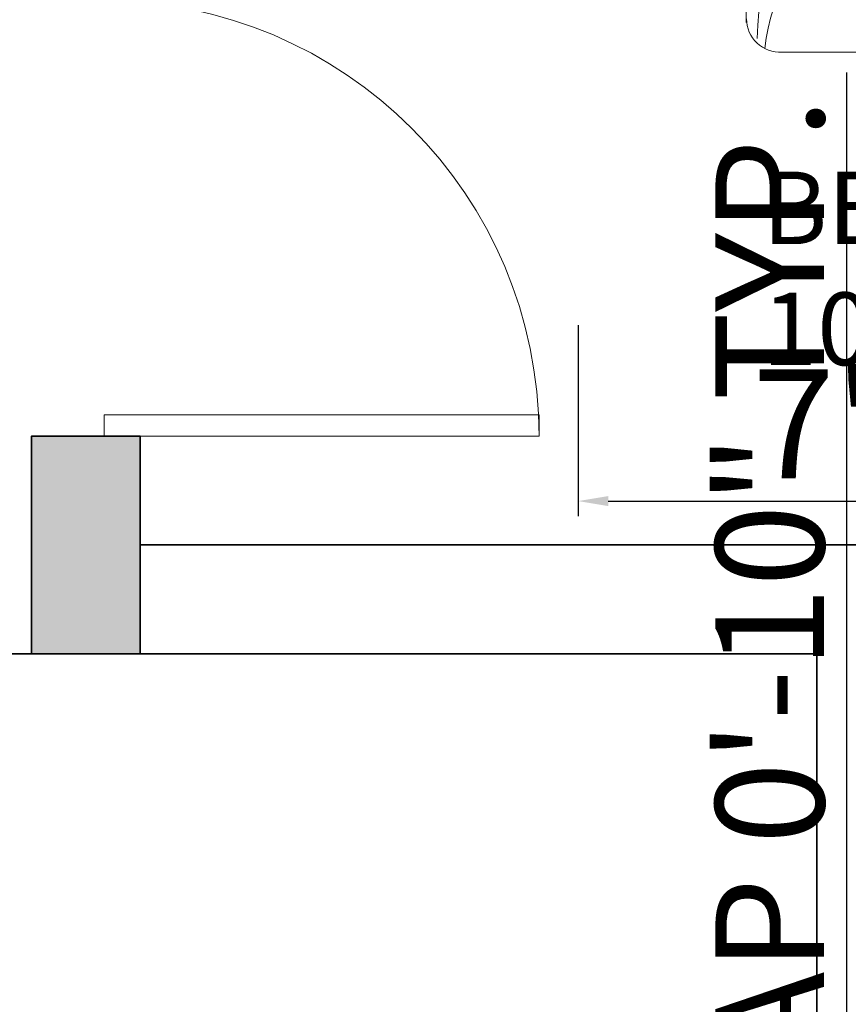
# Model space of a CAD drawing. Units: inches. Extents: x 3321 to 5237, y 11 to 1752.
# Tile 29 of 43: x 4991 to 5060, y 1396 to 1478. Entities that reach past the tile are written whole.
import ezdxf

# ---------------------------------------------------------------- set-up
doc = ezdxf.new("R2010")
doc.units = ezdxf.units.IN
for name, color, linetype, lineweight in [('A-ANNO-DIMS', 2, 'Continuous', 18), ('A-AREA-IDEN', 7, 'Continuous', 18), ('A-COLS', 1, 'Continuous', 35), ('A-DOOR', 4, 'Continuous', 18), ('A-WALL', 7, 'Continuous', 35), ('FUR', 42, 'Continuous', 18)]:
    doc.layers.add(name, color=color, linetype=linetype, lineweight=lineweight)
doc.styles.get("Standard").update_dxf_attribs({"font": 'arial.ttf'})
doc.dimstyles.new('ISO-25', dxfattribs={"dimtxt": 9, "dimasz": 2.5, "dimexe": 1.25, "dimexo": 0.625, "dimtad": 1, "dimdec": 1, "dimlunit": 3, "dimtxsty": 'Standard', "dimcen": 2.5, "dimclrd": 4, "dimclre": 4, "dimclrt": 256, "dimadec": 0, "dimazin": 0, "dimtfac": 1, "dimtdec": 1, "dimtmove": 0, "dimatfit": 3, "dimfxl": 1, "dimarcsym": 0})

# ---------------------------------------------------------------- blocks, each defined once
blk = doc.blocks.new('*U4')
for p, q in [((0, 0), (0, -6)), ((-36, 0), (-36, -6))]:
    blk.add_line(p, q)
blk.add_lwpolyline([(0, 0), (0, 36), (-1.75, 36), (-1.75, 0)], close=True)
blk.add_arc((0, 0), 36, 90, 180)
blk = doc.blocks.new('*X127')
at = {"color": 0}
for p, q in [((3155.9, 8182.9), (3155.9, 8182.9)), ((3147.8, 8143.4), (3147.8, 8143.4)), ((3283, 8049.6), (3283, 8049.6)), ((3209.5, 8023.9), (3209.5, 8023.9)), ((3251.6, 7997), (3251.6, 7997)), ((3154.1, 7950.7), (3154.1, 7950.7))]:
    blk.add_line(p, q, dxfattribs=at)
blk = doc.blocks.new('*X126')
at = {"color": 0}
for p, q in [((3155.9, 8182.9), (3155.9, 8182.9)), ((3139.8, 7939.7), (3139.8, 7939.7))]:
    blk.add_line(p, q, dxfattribs=at)
blk = doc.blocks.new('*X125')
at = {"color": 0}
for p, q in [((3155.9, 8182.9), (3155.9, 8182.9)), ((3139.8, 7939.7), (3139.8, 7939.7))]:
    blk.add_line(p, q, dxfattribs=at)
blk = doc.blocks.new('*X124')
at = {"color": 0}
for p, q in [((3163, 7776.2), (3163, 7776.2)), ((3422.2, 7761.3), (3422.2, 7761.3)), ((3244.3, 7698.6), (3244.3, 7698.6)), ((3340.3, 7689.4), (3340.3, 7689.4)), ((3236.2, 7675.7), (3236.2, 7675.7))]:
    blk.add_line(p, q, dxfattribs=at)
blk = doc.blocks.new('BED1')
for p, q in [((0, -1000), (0, 800)), ((150, 800), (0, 800)), ((150, 800), (150, -1000)), ((2058.7, 800), (150, 800)), ((528, 800), (528, -1000)), ((211.8, 614.9), (277.5, 585.4)), ((2537.2, 404.9), (2237.2, 404.9)), ((2187.2, 354.9), (2187.2, -545.1)), ((2587.2, -545.1), (2587.2, 354.9)), ((2582, 188.1), (2565.4, 174.8)), ((2566.3, 178.5), (2565.2, 177.4)), ((2565.4, 174.8), (2585.7, 165.4)), ((2566.3, -296.8), (2565.2, -297.9)), ((2582, -287.1), (2565.4, -300.5)), ((2565.4, -300.5), (2585.7, -309.9)), ((2237.2, -595.1), (2537.2, -595.1)), ((150, -1000), (0, -1000)), ((150, -1000), (2063.5, -1000))]:
    blk.add_line(p, q)
for points in [[(934, 797.9), (930.9, 797.7), (928.3, 797.4), (926.3, 796.9), (924.9, 796.3), (923.8, 795.6), (923.1, 794.8), (922.7, 793.8), (922.5, 792.7), (922.4, 791.5), (922.5, 790.3), (922.6, 789.2), (922.6, 788.3), (922.6, 787.6), (922.4, 787.3), (922, 787.4), (921.4, 787.9), (920.6, 788.9), (919.5, 790.2), (918.4, 791.6), (917.1, 793.1), (915.9, 794.6), (914.6, 796), (913.3, 797.1), (912.2, 797.9), (911.1, 798.3), (910.1, 798.4), (909.2, 798), (908.3, 797.1), (907.5, 795.8), (906.8, 793.9), (906, 791.4), (905.4, 788.5), (904.8, 785.2), (904.2, 781.7), (903.7, 778.4), (903.2, 775.4), (902.8, 772.9), (902.5, 771.3), (902.3, 770.6), (902.1, 771.2), (902, 772.8), (901.8, 775.2), (901.7, 778.1), (901.5, 781.5), (901.2, 785), (900.8, 788.4), (900.2, 791.5), (899.5, 794.1), (898.6, 796.2), (897.6, 797.9), (896.5, 799.2), (895.3, 800), (894.1, 800.5), (893, 800.7), (891.9, 800.5), (890.9, 800.1), (890, 799), (889.1, 797.1), (888.3, 794), (887.6, 789.3), (886.9, 782.9), (886.2, 774.2), (885.5, 763.1), (884.8, 749.5), (884.2, 734.2), (883.6, 718.3), (883, 702.8), (882.5, 688.8), (882, 677.5), (881.7, 669.8), (881.5, 666.9), (881.3, 669.4), (881.3, 676.7), (881.3, 687.8), (881.2, 701.5), (881.1, 716.8), (880.8, 732.6), (880.2, 748), (879.4, 761.8), (878.3, 773.2), (876.9, 782.2), (875.1, 789.2), (872.9, 794.4), (870.3, 798), (869, 799)], [(2150, -913.5), (2150, 723.2)], [(2327.6, 182.3), (2530, 185.9), (2550.8, 181.9), (2561.7, 179), (2566, 176.7), (2566.9, 174.4), (2566.3, 171.9), (2562, 169.2), (2550.3, 166.5), (2527.7, 163.9), (2490.6, 161.8), (2345.5, 160.2), (2317.8, 158.5)], [(494.7, 3.1), (458.9, 95.3)], [(2149.7, -259.9), (2150, -268.4), (2150.1, -274.1), (2150.1, -278.1), (2150, -281.4), (2149.8, -284), (2149.5, -286.1), (2149.1, -287.8), (2148.7, -289), (2148.1, -289.9), (2147.4, -290.5), (2146.6, -290.8), (2145.6, -291), (2144.6, -291), (2143.6, -291), (2142.7, -290.9), (2141.9, -290.9), (2141.4, -290.9), (2141.1, -291), (2141.2, -291.4), (2141.7, -291.9), (2142.5, -292.6), (2143.5, -293.4), (2144.7, -294.4), (2146, -295.4), (2147.2, -296.5), (2148.4, -297.6), (2149.3, -298.6), (2150, -299.6), (2150.3, -300.5), (2150.4, -301.3), (2150, -302.1), (2149.3, -302.8), (2148.2, -303.5), (2146.6, -304.1), (2144.6, -304.7), (2142.1, -305.2), (2139.3, -305.7), (2136.5, -306.2), (2133.7, -306.6), (2131.2, -307), (2129.2, -307.3), (2127.8, -307.6), (2127.3, -307.8), (2127.7, -308), (2129, -308.1), (2131, -308.2), (2133.5, -308.3), (2136.3, -308.5), (2139.2, -308.7), (2142, -309), (2144.6, -309.5), (2146.8, -310.1), (2148.6, -310.9), (2150, -311.7), (2151, -312.7), (2151.7, -313.6), (2152.1, -314.6), (2152.3, -315.6), (2152.2, -316.5), (2151.8, -317.3), (2150.9, -318.1), (2149.3, -318.8), (2146.7, -319.4), (2142.8, -320), (2137.4, -320.6), (2130.2, -321.2), (2121, -321.8), (2109.7, -322.3), (2096.9, -322.9), (2083.6, -323.4), (2070.7, -323.9), (2059.1, -324.3), (2049.6, -324.7), (2043.2, -325), (2040.8, -325.2), (2042.9, -325.3), (2049, -325.3), (2058.2, -325.3), (2069.6, -325.4), (2082.3, -325.5), (2095.6, -325.8), (2108.4, -326.2), (2119.9, -326.8), (2129.4, -327.8), (2136.9, -329), (2142.7, -330.5), (2147, -332.3), (2150, -334.4), (2150.9, -335.6)], [(2246.5, -294.4), (2530, -289.4), (2550.8, -293.4), (2561.7, -296.3), (2566, -298.6), (2566.9, -300.8), (2566.3, -303.4), (2562, -306.1), (2550.3, -308.8), (2527.7, -311.3), (2490.6, -313.5), (2345.5, -315), (2238.6, -321.8)], [(1733.7, -998.3), (1731.1, -998.1), (1729, -997.8), (1727.4, -997.4), (1726.1, -997), (1725.2, -996.4), (1724.7, -995.7), (1724.3, -994.8), (1724.1, -993.9), (1724.1, -992.9), (1724.1, -991.9), (1724.2, -991), (1724.2, -990.2), (1724.2, -989.7), (1724.1, -989.4), (1723.8, -989.5), (1723.2, -990), (1722.5, -990.8), (1721.7, -991.8), (1720.7, -993), (1719.7, -994.3), (1718.6, -995.5), (1717.5, -996.6), (1716.5, -997.6), (1715.5, -998.3), (1714.6, -998.6), (1713.8, -998.6), (1713, -998.3), (1712.3, -997.6), (1711.7, -996.5), (1711, -994.9), (1710.4, -992.9), (1709.9, -990.4), (1709.4, -987.6), (1708.9, -984.8), (1708.5, -982), (1708.1, -979.5), (1707.8, -977.4), (1707.5, -976.1), (1707.3, -975.5), (1707.1, -976), (1707, -977.3), (1706.9, -979.3), (1706.8, -981.8), (1706.7, -984.6), (1706.4, -987.5), (1706.1, -990.3), (1705.6, -992.9), (1705, -995.1), (1704.2, -996.9), (1703.4, -998.3), (1702.4, -999.3), (1701.5, -1000), (1700.5, -1000.4), (1699.6, -1000.6), (1698.7, -1000.4), (1697.8, -1000.1), (1697, -999.2), (1696.3, -997.6), (1695.7, -995), (1695.1, -991.1), (1694.5, -985.7), (1693.9, -978.5), (1693.3, -969.3), (1692.8, -957.9), (1692.2, -945.2), (1691.7, -931.9), (1691.2, -919), (1690.8, -907.4), (1690.4, -897.9), (1690.1, -891.5), (1689.9, -889.1), (1689.8, -891.2), (1689.8, -897.3), (1689.8, -906.5), (1689.7, -917.9), (1689.6, -930.6), (1689.4, -943.8), (1688.9, -956.6), (1688.3, -968.1), (1687.3, -977.6), (1686.1, -985.2), (1684.6, -991), (1682.8, -995.3), (1680.7, -998.3), (1679.6, -999.2)]]:
    blk.add_lwpolyline(points)
for points in [[(205.5, 619.6, 0.267769), (215.1, 582.4, -0.037739), (204.3, 21.8, 0.684696), (236.7, 5.5, -0.060702), (497.2, 0.1, -0.046649), (225.9, 3.1, -1.318436)], [(489.2, 619.6, 0.144019), (207.6, 617.9, 0.248643)], [(497.2, 0.1, 0.021276), (489.2, 619.6, -0.206383), (326.6, 509.4, 0.237198)], [(211.8, 12.8, 0.143972), (361.6, 262.9, 1.292232)], [(886.4, -150, -0.069098), (985, -66.5, 0.658965), (982.1, -48.7, -0.049789), (927.4, -29, -0.103757), (896.6, -5.4, 0.055725), (800.9, 83.3, -0.11866), (782.7, 104.9, 0.016811), (761.6, 143.9, 0.70791), (748.3, 144, -0.16964), (551.9, -96.6, 0.664036), (554, -110.7, 0.023706), (627, -144.7, -0.134834), (683.2, -188, 0.012748), (746.3, -267.4)], [(969.1, -259.1, 0.263265), (936.3, -236.9, -0.026108), (909.2, -233.2, 0.027613), (945.1, -234.2, -0.089259), (872.7, -120, 0.662242), (857.6, -119.3, -0.162037), (651.8, -332.7, 0.676499), (654, -354.5, -0.160513), (722.9, -401.5, 0.07473), (773.5, -450.3, -0.187721), (845.5, -559.9, 0.70791), (858.8, -561.4, -0.010003), (898.6, -497.3, -0.113819), (947.3, -450.2, 0.099539), (1032.5, -372.4, -0.173425), (1070.9, -346.4, 0.589988), (1076.2, -326.1, 0.137312), (923.9, -245.9, 0.137312)], [(489.2, -168.2, 0.144019), (207.6, -169.9, 0.248643)], [(205.5, -168.2, 0.267769), (215.1, -205.4, -0.037739), (204.3, -766, 0.684696), (236.7, -782.3, -0.060702), (497.2, -787.7, -0.046649), (225.9, -784.7, -1.318436)], [(497.2, -787.7, 0.021276), (489.2, -168.2, -0.206383), (326.6, -278.4, 0.237198)], [(1446, -733.4, -0.095039), (652.8, -1001.7)]]:
    blk.add_lwpolyline(points, format="xyb")
for centre, radius, start, end in [((3208.8, 1363.3), 2739.4, 191.8679, 206.3247), ((2062.7, 713.7), 86.5, 0, 93.5376), ((1608.1, 842.5), 496.3, 305.1901, 354.0206), ((1138.6, 793.9), 983.2, 294.6078, 358.3033), ((2237.2, 354.9), 50, 90, 180), ((2321.1, 409.7), 84.5, 185.6196, 217.1396), ((2227.5, 373.5), 32.8, 17.833, 72.8005), ((2546.9, 373.5), 32.8, 107.1995, 162.167), ((2453.3, 409.7), 84.5, 322.8604, 354.3804), ((2537.2, 354.9), 50, 0, 90), ((2098.7, 754.7), 1625, 193.905, 207.8169), ((2201.9, 323.3), 34.8, 50.8413, 114.9586), ((2212.2, 381.5), 36.5, 226.8095, 258.3841), ((2572.5, 323.3), 34.8, 65.0414, 129.1587), ((2562.2, 381.5), 36.5, 281.6159, 313.1905), ((751.8, 88.7), 34.9, 336.8352, 27.7218), ((684.2, 86), 100.3, 353.675, 10.882), ((1074.1, 198.8), 306.1, 197.8602, 241.5122), ((341.4, -277.7), 318.5, 60.7125, 115.009), ((983.7, -79.5), 20.8, 73.7967, 130.4566), ((978.5, -68.6), 14.3, 39.7097, 85.9506), ((602.5, -324), 198.6, 43.2035, 95.0556), ((3208.8, 1363.3), 2739.4, 212.9314, 216.951), ((981.1, -281.8), 131.1, 164.0372, 243.4536), ((980, -379), 163.4, 152.6104, 209.361), ((3208.8, 1363.3), 2739.4, 218.6329, 229.9449), ((2098.7, 754.7), 1625, 226.5887, 246.3156), ((3402.5, -342.9), 1408.5, 182.9917, 205.6819), ((-34.4, -471.2), 376.5, 312.0118, 350.9635), ((2178, -513.5), 33, 286.1827, 338.1386), ((2188.1, -476.2), 73, 269.4513, 322.8027), ((2562.2, -571.8), 36.5, 46.8095, 78.3841), ((2237.2, -545.1), 50, 180, 270), ((2271.1, -580.9), 35.8, 148.9055, 197.5541), ((2453.3, -600), 84.5, 5.6196, 37.1396), ((2537.2, -545.1), 50, 270, 0), ((2572.5, -513.6), 34.8, 230.8413, 294.9586), ((2546.9, -563.8), 32.8, 197.833, 252.8005), ((375.7, -807.4), 128.2, 17.4073, 88.5129), ((341.4, -1065.5), 318.5, 60.7125, 115.009), ((1929.1, -1126), 250.5, 37.8553, 88.4405), ((2063.5, -913.5), 86.5, 270, 0)]:
    blk.add_arc(centre, radius, start, end)
for name in ['*X126', '*X125', '*X127', '*X124']:
    blk.add_blockref(name, (-2425.3, -8101.4))
blk = doc.blocks.new('A$C68AE1801')
at = {"layer": 'FUR', "xscale": 0.001, "yscale": 0.001, "zscale": 0.001, "rotation": 180}
blk.add_blockref('BED1', (2.5872, 1.49), dxfattribs=at)
blk = doc.blocks.new('COL-9X18-IN')
h = blk.add_hatch(color=256)
h.dxf.hatch_style = 1
h.paths.add_polyline_path([(9, 18), (0, 18), (0, 0), (9, 0)])
blk.add_lwpolyline([(0, 0), (9, 0), (9, 18), (0, 18)], close=True)
blk = doc.blocks.new('*D194')
at = {"layer": 'A-ANNO-DIMS', "color": 4, "lineweight": -2, "transparency": 16777216}
for p, q in [((5037.321, 1452.516), (5037.321, 1436.712)), ((5121.084, 1452.516), (5121.084, 1436.712)), ((5039.821, 1437.962), (5118.584, 1437.962))]:
    blk.add_line(p, q, dxfattribs=at)
at = {"layer": 'A-ANNO-DIMS', "color": 4, "transparency": 16777216}
for points in [[(5039.821, 1438.379), (5039.821, 1437.545), (5037.321, 1437.962)], [(5118.584, 1438.379), (5118.584, 1437.545), (5121.084, 1437.962)]]:
    blk.add_solid(points, dxfattribs=at)
at = {"layer": 'Defpoints', "color": 0, "transparency": 16777216}
for p in [(5037.321, 1453.141), (5121.084, 1453.141), (5121.084, 1437.962)]:
    blk.add_point(p, dxfattribs=at)
at = {"layer": 'A-ANNO-DIMS', "transparency": 16777216, "insert": (5079.203, 1443.182), "char_height": 9, "attachment_point": 5}
blk.add_mtext('7\'-0" TYP.', dxfattribs=at)
blk = doc.blocks.new('*D199')
at = {"layer": 'A-ANNO-DIMS', "color": 4, "lineweight": -2, "transparency": 16777216}
for p, q in [((5059.569, 1379.636), (5059.569, 1473.411)), ((5060.444, 1379.636), (5058.319, 1379.636)), ((5059.569, 1372.136), (5059.569, 1377.136)), ((5060.444, 1369.636), (5058.319, 1369.636))]:
    blk.add_line(p, q, dxfattribs=at)
at = {"layer": 'A-ANNO-DIMS', "color": 4, "transparency": 16777216}
for points in [[(5059.153, 1377.136), (5059.986, 1377.136), (5059.569, 1379.636)], [(5059.153, 1372.136), (5059.986, 1372.136), (5059.569, 1369.636)]]:
    blk.add_solid(points, dxfattribs=at)
at = {"layer": 'Defpoints', "color": 0, "transparency": 16777216}
for p in [(5059.569, 1379.636), (5061.069, 1379.636), (5061.069, 1369.636)]:
    blk.add_point(p, dxfattribs=at)
at = {"layer": 'A-ANNO-DIMS', "transparency": 16777216, "insert": (5054.349, 1427.773), "char_height": 9, "attachment_point": 5, "rotation": 90}
blk.add_mtext('TAP 0\'-10" TYP.', dxfattribs=at)

msp = doc.modelspace()

# ---------------------------------------------------------------- linework, layer by layer
at = {"layer": 'A-WALL'}
for p, q in [((4992.084, 1443.339), (5001.084, 1443.339)), ((5001.084, 1443.339), (5001.084, 1434.339)), ((5001.084, 1434.339), (5087.084, 1434.339)), ((4940.084, 1425.339), (5057.084, 1425.339)), ((5057.084, 1425.339), (5057.084, 1375.339))]:
    msp.add_line(p, q, dxfattribs=at)

# ---------------------------------------------------------------- block references
at = {"layer": 'A-COLS', "rotation": 180}
msp.add_blockref('COL-9X18-IN', (5001.084, 1443.339), dxfattribs=at)
at = {"layer": 'A-DOOR', "rotation": 270}
msp.add_blockref('*U4', (4998.084, 1443.339), dxfattribs=at)
at = {"layer": 'FUR', "xscale": 31.82298296329056, "yscale": 31.82298296329056, "zscale": 31.82298296329056}
msp.add_blockref('A$C68AE1801', (5037.321, 1453.141), dxfattribs=at)

# ---------------------------------------------------------------- texts
at = {"layer": 'A-AREA-IDEN', "insert": (5052.569, 1465.211), "char_height": 6, "attachment_point": 1}
msp.add_mtext_dynamic_manual_height_columns('BEDROOM\\P10\'0"X10\'0"', width=97.3114, gutter_width=25, heights=[0], dxfattribs=at)

# ---------------------------------------------------------------- dimensions: what is measured, and where the dimension line sits
at = {"layer": 'A-ANNO-DIMS'}
dim = msp.add_linear_dim(base=(5059.569, 1379.636), p1=(5061.069, 1369.636), p2=(5061.069, 1379.636), angle=90, text='TAP <> TYP.', dimstyle='ISO-25', override={"dimdec": 1, "dimlfac": 1, "dimrnd": 0, "dimzin": 1, "dimdsep": 46, "dimlunit": 4, "dimfrac": 2}, dxfattribs=at)
dim.commit()
dim.dimension.update_dxf_attribs({"geometry": '*D199', "text_midpoint": (5054.349, 1427.773)})
dim = msp.add_linear_dim(base=(5121.084, 1437.962), p1=(5037.321, 1453.141), p2=(5121.084, 1453.141), text='<> TYP.', dimstyle='ISO-25', override={"dimdec": 1, "dimlfac": 1, "dimrnd": 0, "dimzin": 1, "dimdsep": 46, "dimlunit": 4, "dimfrac": 2}, dxfattribs=at)
dim.commit()
dim.dimension.update_dxf_attribs({"geometry": '*D194', "text_midpoint": (5079.203, 1443.182)})

doc.saveas('drawing.dxf')
